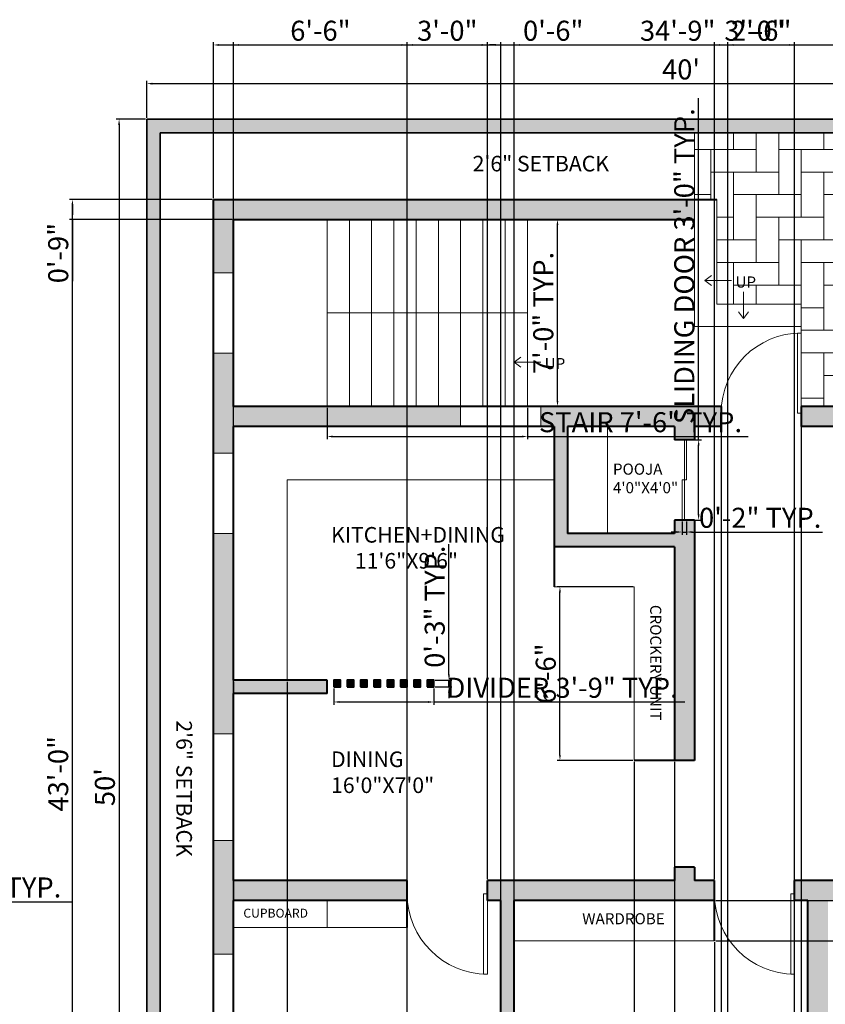
# Model space of a CAD drawing. Units: inches. Extents: x 2337 to 3570, y 1258 to 1938.
# Tile 21 of 30: x 2931 to 3293, y 1496 to 1938. Entities that reach past the tile are written whole.
import ezdxf

# ---------------------------------------------------------------- set-up
doc = ezdxf.new("R2010")
doc.units = ezdxf.units.IN
for name, color, linetype, lineweight in [('A-ANNO-DIMS', 2, 'Continuous', 18), ('A-ANNO-SYMB', 7, 'Continuous', 18), ('A-ANNO-TEXT', 7, 'Continuous', 18), ('A-AREA-IDEN', 7, 'Continuous', 18), ('A-DOOR', 4, 'Continuous', 20), ('A-FLOR-CASE', 34, 'Continuous', 18), ('A-FLOR-PATT', 252, 'Continuous', 13), ('A-FLOR-STRS', 7, 'Continuous', 20), ('A-GLAZ', 4, 'Continuous', 18), ('A-WALL', 7, 'Continuous', 40), ('C-PROP', 7, 'Continuous', 35)]:
    doc.layers.add(name, color=color, linetype=linetype, lineweight=lineweight)
doc.layers.add('A-WALL-PATT', color=18, linetype='Continuous', lineweight=13, true_color=0x000000)
doc.layers.add('C-PROP-PATT', color=251, linetype='Continuous', lineweight=13, true_color=0x636466)
doc.styles.get("Standard").update_dxf_attribs({"font": 'arial.ttf'})
doc.dimstyles.new('ISO-25', dxfattribs={"dimtxt": 9, "dimasz": 2.5, "dimexe": 1.25, "dimexo": 0.625, "dimtad": 1, "dimdec": 1, "dimlunit": 3, "dimtxsty": 'Standard', "dimcen": 2.5, "dimadec": 0, "dimazin": 0, "dimtfac": 1, "dimtdec": 1, "dimtmove": 0, "dimatfit": 3, "dimfxl": 1, "dimarcsym": 0})

# ---------------------------------------------------------------- blocks, each defined once
blk = doc.blocks.new('*U2')
for p, q in [((0, 0), (0, -6)), ((36, 0), (36, -6))]:
    blk.add_line(p, q)
blk.add_lwpolyline([(0, 0), (0, 36), (1.75, 36), (1.75, 0)], close=True)
blk.add_arc((0, 0), 36, 0, 90)
blk = doc.blocks.new('*D4')
at = {"layer": 'A-ANNO-DIMS', "color": 0, "lineweight": -2, "transparency": 16777216}
for p, q in [((2987.79, 1893.74), (2987.79, 1910.39)), ((2990.29, 1909.14), (3465.29, 1909.14)), ((3467.79, 1893.74), (3467.79, 1910.39))]:
    blk.add_line(p, q, dxfattribs=at)
at = {"layer": 'A-ANNO-DIMS', "color": 0, "transparency": 16777216}
for points in [[(2990.29, 1909.55), (2990.29, 1908.72), (2987.79, 1909.14)], [(3465.29, 1909.55), (3465.29, 1908.72), (3467.79, 1909.14)]]:
    blk.add_solid(points, dxfattribs=at)
at = {"layer": 'Defpoints', "color": 0, "transparency": 16777216}
for p in [(3467.79, 1909.14), (2987.79, 1893.12), (3467.79, 1893.12)]:
    blk.add_point(p, dxfattribs=at)
at = {"layer": 'A-ANNO-DIMS', "color": 0, "transparency": 16777216, "insert": (3227.79, 1914.36), "char_height": 9, "attachment_point": 5}
blk.add_mtext("40'", dxfattribs=at)
blk = doc.blocks.new('*D5')
at = {"layer": 'A-ANNO-DIMS', "color": 0, "lineweight": -2, "transparency": 16777216}
for p, q in [((2987.16, 1893.12), (2974.1, 1893.12)), ((2975.35, 1890.62), (2975.35, 1295.62)), ((2987.16, 1293.12), (2974.1, 1293.12))]:
    blk.add_line(p, q, dxfattribs=at)
at = {"layer": 'A-ANNO-DIMS', "color": 0, "transparency": 16777216}
for points in [[(2974.93, 1890.62), (2975.77, 1890.62), (2975.35, 1893.12)], [(2974.93, 1295.62), (2975.77, 1295.62), (2975.35, 1293.12)]]:
    blk.add_solid(points, dxfattribs=at)
at = {"layer": 'Defpoints', "color": 0, "transparency": 16777216}
for p in [(2987.79, 1893.12), (2975.35, 1293.12), (2987.79, 1293.12)]:
    blk.add_point(p, dxfattribs=at)
at = {"layer": 'A-ANNO-DIMS', "color": 0, "transparency": 16777216, "insert": (2970.13, 1593.12), "char_height": 9, "attachment_point": 5, "rotation": 90}
blk.add_mtext("50'", dxfattribs=at)
blk = doc.blocks.new('STAIR-UP-ARROW')
for p, q in [((2.25, 12), (2.25, 0)), ((2.25, 0), (0, 3.01)), ((2.25, 0), (4.5, 3.01))]:
    blk.add_line(p, q)
blk = doc.blocks.new('DOOR-SLIDING-36IN')
for p, q in [((1, 36), (1, 0)), ((2, 18), (2, 36)), ((1, 18), (0, 18)), ((0, 18), (0, 0)), ((1, 18), (2, 18))]:
    blk.add_line(p, q)
blk = doc.blocks.new('STAIR-DOUBLE-FLIGHT')
for p, q in [((0, 0), (0, 84)), ((10, 0), (10, 84)), ((20, 0), (20, 84)), ((30, 0), (30, 84)), ((40, 0), (40, 84)), ((50, 0), (50, 84)), ((60, 0), (60, 84)), ((70, 0), (70, 84)), ((80, 0), (80, 84)), ((90, 0), (90, 84)), ((0, 42), (90, 42))]:
    blk.add_line(p, q)
blk = doc.blocks.new('SCREEN-DIVIDER-8-POST')
h = blk.add_hatch(color=256)
h.dxf.hatch_style = 1
h.paths.add_polyline_path([(3, 3), (0, 3), (0, 0), (3, 0)])
h = blk.add_hatch(color=256)
h.dxf.hatch_style = 1
h.paths.add_polyline_path([(6, 3), (6, 0), (9, 0), (9, 3)])
h = blk.add_hatch(color=256)
h.dxf.hatch_style = 1
h.paths.add_polyline_path([(15, 3), (12, 3), (12, 0), (15, 0)])
h = blk.add_hatch(color=256)
h.dxf.hatch_style = 1
h.paths.add_polyline_path([(18, 3), (18, 0), (21, 0), (21, 3)])
h = blk.add_hatch(color=256)
h.dxf.hatch_style = 1
h.paths.add_polyline_path([(27, 3), (24, 3), (24, 0), (27, 0)])
h = blk.add_hatch(color=256)
h.dxf.hatch_style = 1
h.paths.add_polyline_path([(30, 3), (30, 0), (33, 0), (33, 3)])
h = blk.add_hatch(color=256)
h.dxf.hatch_style = 1
h.paths.add_polyline_path([(39, 3), (36, 3), (36, 0), (39, 0)])
h = blk.add_hatch(color=256)
h.dxf.hatch_style = 1
h.paths.add_polyline_path([(42, 3), (42, 0), (45, 0), (45, 3)])
for points in [[(0, 0), (3, 0), (3, 3), (0, 3)], [(6, 0), (9, 0), (9, 3), (6, 3)], [(12, 0), (15, 0), (15, 3), (12, 3)], [(18, 0), (21, 0), (21, 3), (18, 3)], [(24, 0), (27, 0), (27, 3), (24, 3)], [(30, 0), (33, 0), (33, 3), (30, 3)], [(36, 0), (39, 0), (39, 3), (36, 3)], [(42, 0), (45, 0), (45, 3), (42, 3)]]:
    blk.add_lwpolyline(points, close=True)
blk = doc.blocks.new('*D50')
at = {"layer": 'A-ANNO-DIMS', "color": 0, "lineweight": -2, "transparency": 16777216}
for p, q in [((2777.67, 1538.17), (2777.67, 1542.83)), ((2780.17, 1541.58), (2802.05, 1541.58)), ((2804.55, 1538.17), (2804.55, 1542.83)), ((2804.55, 1541.58), (2954.22, 1541.58))]:
    blk.add_line(p, q, dxfattribs=at)
at = {"layer": 'A-ANNO-DIMS', "color": 0, "transparency": 16777216}
for points in [[(2780.17, 1542), (2780.17, 1541.16), (2777.67, 1541.58)], [(2802.05, 1542), (2802.05, 1541.16), (2804.55, 1541.58)]]:
    blk.add_solid(points, dxfattribs=at)
at = {"layer": 'Defpoints', "color": 0, "transparency": 16777216}
for p in [(2804.55, 1541.58), (2777.67, 1537.55), (2804.55, 1537.55)]:
    blk.add_point(p, dxfattribs=at)
at = {"layer": 'A-ANNO-DIMS', "color": 0, "transparency": 16777216, "insert": (2880.63, 1546.87), "char_height": 9, "attachment_point": 5}
blk.add_mtext('PORCH CHAIR 2\'-3" TYP.', dxfattribs=at)
blk = doc.blocks.new('*D70')
at = {"layer": 'A-ANNO-DIMS', "color": 0, "lineweight": -2, "transparency": 16777216}
for p, q in [((3235.69, 1749.12), (3235.69, 1902.69)), ((3230.91, 1749.12), (3236.94, 1749.12)), ((3235.69, 1715.62), (3235.69, 1746.62)), ((3230.91, 1713.12), (3236.94, 1713.12))]:
    blk.add_line(p, q, dxfattribs=at)
at = {"layer": 'A-ANNO-DIMS', "color": 0, "transparency": 16777216}
for points in [[(3235.27, 1746.62), (3236.1, 1746.62), (3235.69, 1749.12)], [(3235.27, 1715.62), (3236.1, 1715.62), (3235.69, 1713.12)]]:
    blk.add_solid(points, dxfattribs=at)
at = {"layer": 'Defpoints', "color": 0, "transparency": 16777216}
for p in [(3230.29, 1749.12), (3235.69, 1749.12), (3230.29, 1713.12)]:
    blk.add_point(p, dxfattribs=at)
at = {"layer": 'A-ANNO-DIMS', "color": 0, "transparency": 16777216, "insert": (3230.4, 1827.15), "char_height": 9, "attachment_point": 5, "rotation": 90}
blk.add_mtext('SLIDING DOOR 3\'-0" TYP.', dxfattribs=at)
blk = doc.blocks.new('*D71')
at = {"layer": 'A-ANNO-DIMS', "color": 0, "lineweight": -2, "transparency": 16777216}
for p, q in [((3228.29, 1712.49), (3228.29, 1706.47)), ((3230.29, 1712.49), (3230.29, 1706.47)), ((3225.79, 1707.72), (3223.29, 1707.72)), ((3228.29, 1707.72), (3230.29, 1707.72)), ((3232.79, 1707.72), (3291.4, 1707.72))]:
    blk.add_line(p, q, dxfattribs=at)
at = {"layer": 'A-ANNO-DIMS', "color": 0, "transparency": 16777216}
for points in [[(3225.79, 1708.13), (3225.79, 1707.3), (3228.29, 1707.72)], [(3232.79, 1708.13), (3232.79, 1707.3), (3230.29, 1707.72)]]:
    blk.add_solid(points, dxfattribs=at)
at = {"layer": 'Defpoints', "color": 0, "transparency": 16777216}
for p in [(3228.29, 1713.12), (3230.29, 1713.12), (3230.29, 1707.72)]:
    blk.add_point(p, dxfattribs=at)
at = {"layer": 'A-ANNO-DIMS', "color": 0, "transparency": 16777216, "insert": (3263.34, 1712.94), "char_height": 9, "attachment_point": 5}
blk.add_mtext('0\'-2" TYP.', dxfattribs=at)
blk = doc.blocks.new('*D72')
at = {"layer": 'A-ANNO-DIMS', "color": 0, "lineweight": -2, "transparency": 16777216}
for p, q in [((3068.79, 1763.49), (3068.79, 1749.37)), ((3158.79, 1763.49), (3158.79, 1749.37)), ((3071.29, 1750.62), (3156.29, 1750.62)), ((3158.79, 1750.62), (3257.87, 1750.62))]:
    blk.add_line(p, q, dxfattribs=at)
at = {"layer": 'A-ANNO-DIMS', "color": 0, "transparency": 16777216}
for points in [[(3071.29, 1751.03), (3071.29, 1750.2), (3068.79, 1750.62)], [(3156.29, 1751.03), (3156.29, 1750.2), (3158.79, 1750.62)]]:
    blk.add_solid(points, dxfattribs=at)
at = {"layer": 'Defpoints', "color": 0, "transparency": 16777216}
for p in [(3068.79, 1764.12), (3158.79, 1764.12), (3158.79, 1750.62)]:
    blk.add_point(p, dxfattribs=at)
at = {"layer": 'A-ANNO-DIMS', "color": 0, "transparency": 16777216, "insert": (3209.58, 1755.89), "char_height": 9, "attachment_point": 5}
blk.add_mtext('STAIR 7\'-6" TYP.', dxfattribs=at)
blk = doc.blocks.new('*D73')
at = {"layer": 'A-ANNO-DIMS', "color": 0, "lineweight": -2, "transparency": 16777216}
for p, q in [((3159.41, 1848.12), (3173.54, 1848.12)), ((3172.29, 1766.62), (3172.29, 1845.62)), ((3159.41, 1764.12), (3173.54, 1764.12))]:
    blk.add_line(p, q, dxfattribs=at)
at = {"layer": 'A-ANNO-DIMS', "color": 0, "transparency": 16777216}
for points in [[(3171.87, 1845.62), (3172.7, 1845.62), (3172.29, 1848.12)], [(3171.87, 1766.62), (3172.7, 1766.62), (3172.29, 1764.12)]]:
    blk.add_solid(points, dxfattribs=at)
at = {"layer": 'Defpoints', "color": 0, "transparency": 16777216}
for p in [(3158.79, 1848.12), (3172.29, 1848.12), (3158.79, 1764.12)]:
    blk.add_point(p, dxfattribs=at)
at = {"layer": 'A-ANNO-DIMS', "color": 0, "transparency": 16777216, "insert": (3167.07, 1806.12), "char_height": 9, "attachment_point": 5, "rotation": 90}
blk.add_mtext('7\'-0" TYP.', dxfattribs=at)
blk = doc.blocks.new('*D76')
at = {"layer": 'A-ANNO-DIMS', "color": 0, "lineweight": -2, "transparency": 16777216}
for p, q in [((3071.79, 1637.49), (3071.79, 1630.12)), ((3116.79, 1637.49), (3116.79, 1630.12)), ((3074.29, 1631.37), (3114.29, 1631.37)), ((3116.79, 1631.37), (3229.44, 1631.37))]:
    blk.add_line(p, q, dxfattribs=at)
at = {"layer": 'A-ANNO-DIMS', "color": 0, "transparency": 16777216}
for points in [[(3074.29, 1631.78), (3074.29, 1630.95), (3071.79, 1631.37)], [(3114.29, 1631.78), (3114.29, 1630.95), (3116.79, 1631.37)]]:
    blk.add_solid(points, dxfattribs=at)
at = {"layer": 'Defpoints', "color": 0, "transparency": 16777216}
for p in [(3071.79, 1638.12), (3116.79, 1638.12), (3116.79, 1631.37)]:
    blk.add_point(p, dxfattribs=at)
at = {"layer": 'A-ANNO-DIMS', "color": 0, "transparency": 16777216, "insert": (3174.36, 1636.59), "char_height": 9, "attachment_point": 5}
blk.add_mtext('DIVIDER 3\'-9" TYP.', dxfattribs=at)
blk = doc.blocks.new('*D77')
at = {"layer": 'A-ANNO-DIMS', "color": 0, "lineweight": -2, "transparency": 16777216}
for p, q in [((3123.54, 1643.62), (3123.54, 1702.23)), ((3117.41, 1641.12), (3124.79, 1641.12)), ((3123.54, 1638.12), (3123.54, 1641.12)), ((3117.41, 1638.12), (3124.79, 1638.12)), ((3123.54, 1635.62), (3123.54, 1633.12))]:
    blk.add_line(p, q, dxfattribs=at)
at = {"layer": 'A-ANNO-DIMS', "color": 0, "transparency": 16777216}
for points in [[(3123.12, 1643.62), (3123.95, 1643.62), (3123.54, 1641.12)], [(3123.12, 1635.62), (3123.95, 1635.62), (3123.54, 1638.12)]]:
    blk.add_solid(points, dxfattribs=at)
at = {"layer": 'Defpoints', "color": 0, "transparency": 16777216}
for p in [(3116.79, 1641.12), (3123.54, 1641.12), (3116.79, 1638.12)]:
    blk.add_point(p, dxfattribs=at)
at = {"layer": 'A-ANNO-DIMS', "color": 0, "transparency": 16777216, "insert": (3118.31, 1674.17), "char_height": 9, "attachment_point": 5, "rotation": 90}
blk.add_mtext('0\'-3" TYP.', dxfattribs=at)
blk = doc.blocks.new('*D98')
at = {"layer": 'A-ANNO-DIMS', "color": 0, "lineweight": -2, "transparency": 16777216}
for p, q in [((3104.79, 1551.74), (3104.79, 1927.77)), ((3107.29, 1926.52), (3138.29, 1926.52)), ((3140.79, 1551.74), (3140.79, 1927.77))]:
    blk.add_line(p, q, dxfattribs=at)
at = {"layer": 'A-ANNO-DIMS', "color": 0, "transparency": 16777216}
for points in [[(3107.29, 1926.93), (3107.29, 1926.1), (3104.79, 1926.52)], [(3138.29, 1926.93), (3138.29, 1926.1), (3140.79, 1926.52)]]:
    blk.add_solid(points, dxfattribs=at)
at = {"layer": 'Defpoints', "color": 0, "transparency": 16777216}
for p in [(3140.79, 1926.52), (3104.79, 1551.12), (3140.79, 1551.12)]:
    blk.add_point(p, dxfattribs=at)
at = {"layer": 'A-ANNO-DIMS', "color": 0, "transparency": 16777216, "insert": (3122.79, 1931.74), "char_height": 9, "attachment_point": 5}
blk.add_mtext('3\'-0"', dxfattribs=at)
blk = doc.blocks.new('*D99')
at = {"layer": 'A-ANNO-DIMS', "color": 0, "lineweight": -2, "transparency": 16777216}
for p, q in [((3242.79, 1551.74), (3242.79, 1927.77)), ((3245.29, 1926.52), (3276.29, 1926.52)), ((3278.79, 1551.74), (3278.79, 1927.77))]:
    blk.add_line(p, q, dxfattribs=at)
at = {"layer": 'A-ANNO-DIMS', "color": 0, "transparency": 16777216}
for points in [[(3245.29, 1926.93), (3245.29, 1926.1), (3242.79, 1926.52)], [(3276.29, 1926.93), (3276.29, 1926.1), (3278.79, 1926.52)]]:
    blk.add_solid(points, dxfattribs=at)
at = {"layer": 'Defpoints', "color": 0, "transparency": 16777216}
for p in [(3278.79, 1926.52), (3242.79, 1551.12), (3278.79, 1551.12)]:
    blk.add_point(p, dxfattribs=at)
at = {"layer": 'A-ANNO-DIMS', "color": 0, "transparency": 16777216, "insert": (3260.79, 1931.74), "char_height": 9, "attachment_point": 5}
blk.add_mtext('3\'-0"', dxfattribs=at)
blk = doc.blocks.new('*D100')
at = {"layer": 'A-ANNO-DIMS', "color": 0, "lineweight": -2, "transparency": 16777216}
for p, q in [((3248.79, 1422.74), (3248.79, 1927.77)), ((3251.29, 1926.52), (3276.29, 1926.52)), ((3278.79, 1422.74), (3278.79, 1927.77))]:
    blk.add_line(p, q, dxfattribs=at)
at = {"layer": 'A-ANNO-DIMS', "color": 0, "transparency": 16777216}
for points in [[(3251.29, 1926.93), (3251.29, 1926.1), (3248.79, 1926.52)], [(3276.29, 1926.93), (3276.29, 1926.1), (3278.79, 1926.52)]]:
    blk.add_solid(points, dxfattribs=at)
at = {"layer": 'Defpoints', "color": 0, "transparency": 16777216}
for p in [(3278.79, 1926.52), (3248.79, 1422.12), (3278.79, 1422.12)]:
    blk.add_point(p, dxfattribs=at)
at = {"layer": 'A-ANNO-DIMS', "color": 0, "transparency": 16777216, "insert": (3263.79, 1931.74), "char_height": 9, "attachment_point": 5}
blk.add_mtext('2\'-6"', dxfattribs=at)
blk = doc.blocks.new('*D102')
at = {"layer": 'A-ANNO-DIMS', "color": 0, "lineweight": -2, "transparency": 16777216}
for p, q in [((3245.79, 1763.49), (3245.79, 1258.47)), ((3281.79, 1763.49), (3281.79, 1258.47)), ((3248.29, 1259.72), (3279.29, 1259.72))]:
    blk.add_line(p, q, dxfattribs=at)
at = {"layer": 'A-ANNO-DIMS', "color": 0, "transparency": 16777216}
for points in [[(3248.29, 1260.13), (3248.29, 1259.3), (3245.79, 1259.72)], [(3279.29, 1260.13), (3279.29, 1259.3), (3281.79, 1259.72)]]:
    blk.add_solid(points, dxfattribs=at)
at = {"layer": 'Defpoints', "color": 0, "transparency": 16777216}
for p in [(3245.79, 1764.12), (3281.79, 1764.12), (3281.79, 1259.72)]:
    blk.add_point(p, dxfattribs=at)
at = {"layer": 'A-ANNO-DIMS', "color": 0, "transparency": 16777216, "insert": (3263.79, 1264.94), "char_height": 9, "attachment_point": 5}
blk.add_mtext('3\'-0"', dxfattribs=at)
blk = doc.blocks.new('*D103')
at = {"layer": 'A-ANNO-DIMS', "color": 0, "lineweight": -2, "transparency": 16777216}
for p, q in [((3017.16, 1857.12), (2953.14, 1857.12)), ((2954.39, 1854.62), (2954.39, 1850.62)), ((3026.16, 1848.12), (2953.14, 1848.12)), ((2954.39, 1848.12), (2954.39, 1820.44))]:
    blk.add_line(p, q, dxfattribs=at)
at = {"layer": 'A-ANNO-DIMS', "color": 0, "transparency": 16777216}
for points in [[(2953.97, 1854.62), (2954.8, 1854.62), (2954.39, 1857.12)], [(2953.97, 1850.62), (2954.8, 1850.62), (2954.39, 1848.12)]]:
    blk.add_solid(points, dxfattribs=at)
at = {"layer": 'Defpoints', "color": 0, "transparency": 16777216}
for p in [(3017.79, 1857.12), (2954.39, 1848.12), (3026.79, 1848.12)]:
    blk.add_point(p, dxfattribs=at)
at = {"layer": 'A-ANNO-DIMS', "color": 0, "transparency": 16777216, "insert": (2949.17, 1833.03), "char_height": 9, "attachment_point": 5, "rotation": 90}
blk.add_mtext('0\'-9"', dxfattribs=at)
blk = doc.blocks.new('*D104')
at = {"layer": 'A-ANNO-DIMS', "color": 0, "lineweight": -2, "transparency": 16777216}
for p, q in [((3144.29, 1926.52), (3141.79, 1926.52)), ((3146.79, 1350.74), (3146.79, 1927.77)), ((3146.79, 1926.52), (3152.79, 1926.52)), ((3152.79, 1350.74), (3152.79, 1927.77)), ((3155.29, 1926.52), (3182.96, 1926.52))]:
    blk.add_line(p, q, dxfattribs=at)
at = {"layer": 'A-ANNO-DIMS', "color": 0, "transparency": 16777216}
for points in [[(3144.29, 1926.93), (3144.29, 1926.1), (3146.79, 1926.52)], [(3155.29, 1926.93), (3155.29, 1926.1), (3152.79, 1926.52)]]:
    blk.add_solid(points, dxfattribs=at)
at = {"layer": 'Defpoints', "color": 0, "transparency": 16777216}
for p in [(3152.79, 1926.52), (3146.79, 1350.12), (3152.79, 1350.12)]:
    blk.add_point(p, dxfattribs=at)
at = {"layer": 'A-ANNO-DIMS', "color": 0, "transparency": 16777216, "insert": (3170.37, 1931.74), "char_height": 9, "attachment_point": 5}
blk.add_mtext('0\'-6"', dxfattribs=at)
blk = doc.blocks.new('*D105')
at = {"layer": 'A-ANNO-DIMS', "color": 0, "lineweight": -2, "transparency": 16777216}
for p, q in [((3026.79, 1640.49), (3026.79, 1258.47)), ((3050.79, 1640.49), (3050.79, 1258.47)), ((3029.29, 1259.72), (3048.29, 1259.72)), ((3050.79, 1259.72), (3078.61, 1259.72))]:
    blk.add_line(p, q, dxfattribs=at)
at = {"layer": 'A-ANNO-DIMS', "color": 0, "transparency": 16777216}
for points in [[(3029.29, 1260.13), (3029.29, 1259.3), (3026.79, 1259.72)], [(3048.29, 1260.13), (3048.29, 1259.3), (3050.79, 1259.72)]]:
    blk.add_solid(points, dxfattribs=at)
at = {"layer": 'Defpoints', "color": 0, "transparency": 16777216}
for p in [(3026.79, 1641.12), (3050.79, 1641.12), (3050.79, 1259.72)]:
    blk.add_point(p, dxfattribs=at)
at = {"layer": 'A-ANNO-DIMS', "color": 0, "transparency": 16777216, "insert": (3065.95, 1264.94), "char_height": 9, "attachment_point": 5}
blk.add_mtext('2\'-0"', dxfattribs=at)
blk = doc.blocks.new('*D110')
at = {"layer": 'A-ANNO-DIMS', "color": 0, "lineweight": -2, "transparency": 16777216}
for p, q in [((3017.16, 1857.12), (2953.14, 1857.12)), ((2954.39, 1343.62), (2954.39, 1854.62)), ((3017.16, 1341.12), (2953.14, 1341.12))]:
    blk.add_line(p, q, dxfattribs=at)
at = {"layer": 'A-ANNO-DIMS', "color": 0, "transparency": 16777216}
for points in [[(2953.97, 1854.62), (2954.8, 1854.62), (2954.39, 1857.12)], [(2953.97, 1343.62), (2954.8, 1343.62), (2954.39, 1341.12)]]:
    blk.add_solid(points, dxfattribs=at)
at = {"layer": 'Defpoints', "color": 0, "transparency": 16777216}
for p in [(2954.39, 1857.12), (3017.79, 1857.12), (3017.79, 1341.12)]:
    blk.add_point(p, dxfattribs=at)
at = {"layer": 'A-ANNO-DIMS', "color": 0, "transparency": 16777216, "insert": (2949.16, 1599.12), "char_height": 9, "attachment_point": 5, "rotation": 90}
blk.add_mtext('43\'-0"', dxfattribs=at)
blk = doc.blocks.new('*D111')
at = {"layer": 'A-ANNO-DIMS', "color": 0, "lineweight": -2, "transparency": 16777216}
for p, q in [((3017.79, 1857.74), (3017.79, 1927.77)), ((3020.29, 1926.52), (3432.29, 1926.52)), ((3434.79, 1764.74), (3434.79, 1927.77))]:
    blk.add_line(p, q, dxfattribs=at)
at = {"layer": 'A-ANNO-DIMS', "color": 0, "transparency": 16777216}
for points in [[(3020.29, 1926.93), (3020.29, 1926.1), (3017.79, 1926.52)], [(3432.29, 1926.93), (3432.29, 1926.1), (3434.79, 1926.52)]]:
    blk.add_solid(points, dxfattribs=at)
at = {"layer": 'Defpoints', "color": 0, "transparency": 16777216}
for p in [(3434.79, 1926.52), (3017.79, 1857.12), (3434.79, 1764.12)]:
    blk.add_point(p, dxfattribs=at)
at = {"layer": 'A-ANNO-DIMS', "color": 0, "transparency": 16777216, "insert": (3226.29, 1931.74), "char_height": 9, "attachment_point": 5}
blk.add_mtext('34\'-9"', dxfattribs=at)
blk = doc.blocks.new('*D112')
at = {"layer": 'A-ANNO-DIMS', "color": 0, "lineweight": -2, "transparency": 16777216}
for p, q in [((3026.79, 1368.74), (3026.79, 1927.77)), ((3029.29, 1926.52), (3102.29, 1926.52)), ((3104.79, 1368.74), (3104.79, 1927.77))]:
    blk.add_line(p, q, dxfattribs=at)
at = {"layer": 'A-ANNO-DIMS', "color": 0, "transparency": 16777216}
for points in [[(3029.29, 1926.93), (3029.29, 1926.1), (3026.79, 1926.52)], [(3102.29, 1926.93), (3102.29, 1926.1), (3104.79, 1926.52)]]:
    blk.add_solid(points, dxfattribs=at)
at = {"layer": 'Defpoints', "color": 0, "transparency": 16777216}
for p in [(3104.79, 1926.52), (3026.79, 1368.12), (3104.79, 1368.12)]:
    blk.add_point(p, dxfattribs=at)
at = {"layer": 'A-ANNO-DIMS', "color": 0, "transparency": 16777216, "insert": (3065.79, 1931.74), "char_height": 9, "attachment_point": 5}
blk.add_mtext('6\'-6"', dxfattribs=at)
blk = doc.blocks.new('*D114')
at = {"layer": 'A-ANNO-DIMS', "color": 0, "lineweight": -2, "transparency": 16777216}
for p, q in [((3152.79, 1523.49), (3152.79, 1258.47)), ((3242.79, 1523.49), (3242.79, 1258.47)), ((3155.29, 1259.72), (3240.29, 1259.72))]:
    blk.add_line(p, q, dxfattribs=at)
at = {"layer": 'A-ANNO-DIMS', "color": 0, "transparency": 16777216}
for points in [[(3155.29, 1260.13), (3155.29, 1259.3), (3152.79, 1259.72)], [(3240.29, 1260.13), (3240.29, 1259.3), (3242.79, 1259.72)]]:
    blk.add_solid(points, dxfattribs=at)
at = {"layer": 'Defpoints', "color": 0, "transparency": 16777216}
for p in [(3152.79, 1524.12), (3242.79, 1524.12), (3242.79, 1259.72)]:
    blk.add_point(p, dxfattribs=at)
at = {"layer": 'A-ANNO-DIMS', "color": 0, "transparency": 16777216, "insert": (3197.79, 1264.94), "char_height": 9, "attachment_point": 5}
blk.add_mtext('7\'-6"', dxfattribs=at)
blk = doc.blocks.new('*D115')
at = {"layer": 'A-ANNO-DIMS', "color": 0, "lineweight": -2, "transparency": 16777216}
for p, q in [((3243.41, 1542.12), (3502.44, 1542.12)), ((3501.19, 1539.62), (3501.19, 1526.62)), ((3243.41, 1524.12), (3502.44, 1524.12)), ((3501.19, 1524.12), (3501.19, 1497.29))]:
    blk.add_line(p, q, dxfattribs=at)
at = {"layer": 'A-ANNO-DIMS', "color": 0, "transparency": 16777216}
for points in [[(3500.77, 1539.62), (3501.6, 1539.62), (3501.19, 1542.12)], [(3500.77, 1526.62), (3501.6, 1526.62), (3501.19, 1524.12)]]:
    blk.add_solid(points, dxfattribs=at)
at = {"layer": 'Defpoints', "color": 0, "transparency": 16777216}
for p in [(3242.79, 1542.12), (3242.79, 1524.12), (3501.19, 1524.12)]:
    blk.add_point(p, dxfattribs=at)
at = {"layer": 'A-ANNO-DIMS', "color": 0, "transparency": 16777216, "insert": (3495.97, 1509.45), "char_height": 9, "attachment_point": 5, "rotation": 90}
blk.add_mtext('1\'-6"', dxfattribs=at)
blk = doc.blocks.new('*D116')
at = {"layer": 'A-ANNO-DIMS', "color": 0, "lineweight": -2, "transparency": 16777216}
for p, q in [((3206.16, 1683.12), (3172.14, 1683.12)), ((3173.39, 1607.62), (3173.39, 1680.62)), ((3206.16, 1605.12), (3172.14, 1605.12))]:
    blk.add_line(p, q, dxfattribs=at)
at = {"layer": 'A-ANNO-DIMS', "color": 0, "transparency": 16777216}
for points in [[(3172.97, 1680.62), (3173.8, 1680.62), (3173.39, 1683.12)], [(3172.97, 1607.62), (3173.8, 1607.62), (3173.39, 1605.12)]]:
    blk.add_solid(points, dxfattribs=at)
at = {"layer": 'Defpoints', "color": 0, "transparency": 16777216}
for p in [(3173.39, 1683.12), (3206.79, 1683.12), (3206.79, 1605.12)]:
    blk.add_point(p, dxfattribs=at)
at = {"layer": 'A-ANNO-DIMS', "color": 0, "transparency": 16777216, "insert": (3168.17, 1644.12), "char_height": 9, "attachment_point": 5, "rotation": 90}
blk.add_mtext('6\'-6"', dxfattribs=at)
blk = doc.blocks.new('*D117')
at = {"layer": 'A-ANNO-DIMS', "color": 0, "lineweight": -2, "transparency": 16777216}
for p, q in [((3206.79, 1604.49), (3206.79, 1258.47)), ((3224.79, 1604.49), (3224.79, 1258.47)), ((3209.29, 1259.72), (3222.29, 1259.72)), ((3224.79, 1259.72), (3251.61, 1259.72))]:
    blk.add_line(p, q, dxfattribs=at)
at = {"layer": 'A-ANNO-DIMS', "color": 0, "transparency": 16777216}
for points in [[(3209.29, 1260.13), (3209.29, 1259.3), (3206.79, 1259.72)], [(3222.29, 1260.13), (3222.29, 1259.3), (3224.79, 1259.72)]]:
    blk.add_solid(points, dxfattribs=at)
at = {"layer": 'Defpoints', "color": 0, "transparency": 16777216}
for p in [(3206.79, 1605.12), (3224.79, 1605.12), (3224.79, 1259.72)]:
    blk.add_point(p, dxfattribs=at)
at = {"layer": 'A-ANNO-DIMS', "color": 0, "transparency": 16777216, "insert": (3239.45, 1264.94), "char_height": 9, "attachment_point": 5}
blk.add_mtext('1\'-6"', dxfattribs=at)

msp = doc.modelspace()

# ---------------------------------------------------------------- hatches: boundary and pattern name
at = {"layer": 'A-FLOR-PATT'}
h = msp.add_hatch(dxfattribs=at)
h.set_pattern_fill('AR-HBONE', color=256, scale=0.1, angle=45)
h.set_pattern_definition([(90, (-558.681, 0), (-10.16, 10.16), [30.48, -10.16]), (180, (-558.681, 10.16), (-10.16, 10.16), [30.48, -10.16])])
h.paths.add_polyline_path([(3281.79, 1810.12), (3281.79, 1764.12), (3434.79, 1764.12), (3461.79, 1764.12), (3461.79, 1779.12), (3464.79, 1779.12), (3464.79, 1875.12), (3461.79, 1875.12), (3461.79, 1887.12), (3233.79, 1887.12), (3233.79, 1857.12), (3243.79, 1857.12), (3243.79, 1810.12)])
h.paths.add_polyline_path([(3250.98, 1816.17), (3263.22, 1816.17), (3263.22, 1823.8), (3250.98, 1823.8)], flags=24)
h.paths.add_polyline_path([(3317.33, 1858.95), (3370.67, 1858.95), (3370.67, 1885.07), (3317.33, 1885.07)], flags=24)
at = {"layer": 'A-WALL-PATT'}
h = msp.add_hatch(color=256, dxfattribs=at)
h.dxf.hatch_style = 1
h.paths.add_polyline_path([(3233.79, 1857.12), (3017.79, 1857.12), (3017.79, 1824.12), (3026.79, 1824.12), (3026.79, 1848.12), (3233.79, 1848.12)])
h.paths.add_polyline_path([(3128.79, 1764.12), (3026.79, 1764.12), (3026.79, 1788.12), (3017.79, 1788.12), (3017.79, 1743.12), (3026.79, 1743.12), (3026.79, 1755.12), (3128.79, 1755.12)])
h.paths.add_polyline_path([(3245.79, 1761.12), (3245.79, 1764.12), (3164.79, 1764.12), (3164.79, 1755.12), (3170.79, 1755.12), (3170.79, 1701.12), (3224.79, 1701.12), (3224.79, 1605.12), (3233.79, 1605.12), (3233.79, 1713.12), (3224.79, 1713.12), (3224.79, 1707.12), (3176.79, 1707.12), (3176.79, 1755.12), (3224.79, 1755.12), (3224.79, 1749.12), (3233.79, 1749.12), (3233.79, 1755.12), (3245.79, 1755.12)])
h.paths.add_polyline_path([(3026.79, 1707.12), (3017.79, 1707.12), (3017.79, 1617.12), (3026.79, 1617.12), (3026.79, 1635.12), (3068.79, 1635.12), (3068.79, 1641.12), (3026.79, 1641.12)])
h.paths.add_polyline_path([(3104.79, 1551.12), (3026.79, 1551.12), (3026.79, 1569.12), (3017.79, 1569.12), (3017.79, 1518.12), (3026.79, 1518.12), (3026.79, 1542.12), (3104.79, 1542.12)])
h.paths.add_polyline_path([(3026.79, 1482.12), (3017.79, 1482.12), (3017.79, 1410.12), (3026.79, 1410.12)])
h.paths.add_polyline_path([(3188.79, 1350.12), (3152.79, 1350.12), (3152.79, 1380.12), (3146.79, 1380.12), (3146.79, 1350.12), (3026.79, 1350.12), (3026.79, 1374.12), (3017.79, 1374.12), (3017.79, 1341.12), (3188.79, 1341.12)])
h.paths.add_polyline_path([(3224.79, 1416.12), (3248.79, 1416.12), (3248.79, 1422.12), (3152.79, 1422.12), (3152.79, 1542.12), (3242.79, 1542.12), (3242.79, 1551.12), (3233.79, 1551.12), (3233.79, 1557.12), (3224.79, 1557.12), (3224.79, 1551.12), (3140.79, 1551.12), (3140.79, 1542.12), (3146.79, 1542.12), (3146.79, 1410.12), (3152.79, 1410.12), (3152.79, 1416.12), (3218.79, 1416.12), (3218.79, 1350.12), (3212.79, 1350.12), (3212.79, 1341.12), (3293.79, 1341.12), (3293.79, 1362.12), (3284.79, 1362.12), (3284.79, 1350.12), (3224.79, 1350.12)])
h.paths.add_polyline_path([(3293.79, 1434.12), (3284.79, 1434.12), (3284.79, 1422.12), (3278.79, 1422.12), (3278.79, 1416.12), (3284.79, 1416.12), (3284.79, 1386.12), (3293.79, 1386.12)], flags=17)
h.paths.add_polyline_path([(3293.79, 1542.12), (3314.79, 1542.12), (3314.79, 1551.12), (3278.79, 1551.12), (3278.79, 1545.12), (3278.79, 1542.12), (3284.79, 1542.12), (3284.79, 1482.12), (3293.79, 1482.12)])
h.paths.add_polyline_path([(3371.79, 1551.12), (3350.79, 1551.12), (3350.79, 1542.12), (3371.79, 1542.12), (3371.79, 1548.12)])
h.paths.add_polyline_path([(3434.79, 1647.12), (3425.79, 1647.12), (3425.79, 1551.12), (3419.79, 1551.12), (3419.79, 1548.12), (3419.79, 1542.12), (3434.79, 1542.12)])
h.paths.add_polyline_path([(3434.79, 1764.12), (3389.79, 1764.12), (3389.79, 1755.12), (3425.79, 1755.12), (3425.79, 1719.12), (3434.79, 1719.12)])
h.paths.add_polyline_path([(3317.79, 1764.12), (3281.79, 1764.12), (3281.79, 1755.12), (3317.79, 1755.12)])
at = {"layer": 'C-PROP-PATT'}
h = msp.add_hatch(color=256, dxfattribs=at)
h.dxf.hatch_style = 1
h.paths.add_polyline_path([(3467.79, 1893.12), (2987.79, 1893.12), (2987.79, 1293.12), (3293.79, 1293.12), (3293.79, 1299.12), (2993.79, 1299.12), (2993.79, 1887.12), (3461.79, 1887.12), (3461.79, 1875.12), (3467.79, 1875.12)])
h.paths.add_polyline_path([(3407.79, 1299.12), (3389.79, 1299.12), (3389.79, 1293.12), (3407.79, 1293.12)], flags=17)
h.paths.add_polyline_path([(3461.79, 1299.12), (3455.79, 1299.12), (3455.79, 1293.12), (3467.79, 1293.12), (3467.79, 1779.12), (3461.79, 1779.12)], flags=17)

# ---------------------------------------------------------------- linework, layer by layer
at = {"layer": 'A-FLOR-CASE'}
for p, q in [((3194.79, 1755.12), (3194.79, 1707.12)), ((3050.79, 1641.12), (3050.79, 1731.12)), ((3170.79, 1731.12), (3050.79, 1731.12)), ((3206.79, 1683.12), (3170.79, 1683.12)), ((3206.79, 1683.12), (3206.79, 1605.12)), ((3068.79, 1530.12), (3068.79, 1542.12)), ((3104.79, 1530.12), (3026.79, 1530.12)), ((3242.79, 1524.12), (3152.79, 1524.12))]:
    msp.add_line(p, q, dxfattribs=at)
at = {"layer": 'A-FLOR-STRS'}
for p, q in [((3233.79, 1887.12), (3233.79, 1800.12)), ((3243.79, 1857.12), (3243.79, 1810.12)), ((3281.79, 1810.12), (3243.79, 1810.12)), ((3281.79, 1764.12), (3281.79, 1810.12)), ((3281.79, 1800.12), (3233.79, 1800.12))]:
    msp.add_line(p, q, dxfattribs=at)
at = {"layer": 'A-GLAZ'}
for p, q in [((3026.79, 1824.12), (3017.79, 1824.12)), ((3026.79, 1788.12), (3017.79, 1788.12)), ((3128.79, 1764.12), (3128.79, 1755.12)), ((3164.79, 1764.12), (3164.79, 1755.12)), ((3026.79, 1743.12), (3017.79, 1743.12)), ((3026.79, 1707.12), (3017.79, 1707.12)), ((3026.79, 1617.12), (3017.79, 1617.12)), ((3026.79, 1569.12), (3017.79, 1569.12)), ((3026.79, 1518.12), (3017.79, 1518.12))]:
    msp.add_line(p, q, dxfattribs=at)
at = {"layer": 'A-WALL'}
for p, q in [((3017.79, 1857.12), (3243.79, 1857.12)), ((3017.79, 1341.12), (3017.79, 1857.12)), ((3026.79, 1848.12), (3233.79, 1848.12)), ((3026.79, 1764.12), (3026.79, 1848.12)), ((3245.79, 1764.12), (3026.79, 1764.12)), ((3245.79, 1764.12), (3245.79, 1755.12)), ((3434.79, 1764.12), (3281.79, 1764.12)), ((3281.79, 1764.12), (3281.79, 1755.12)), ((3026.79, 1641.12), (3026.79, 1755.12)), ((3170.79, 1755.12), (3026.79, 1755.12)), ((3170.79, 1755.12), (3170.79, 1683.12)), ((3176.79, 1755.12), (3176.79, 1707.12)), ((3224.79, 1755.12), (3176.79, 1755.12)), ((3224.79, 1755.12), (3224.79, 1749.12)), ((3233.79, 1755.12), (3233.79, 1749.12)), ((3245.79, 1755.12), (3233.79, 1755.12)), ((3425.79, 1755.12), (3281.79, 1755.12)), ((3233.79, 1749.12), (3224.79, 1749.12)), ((3233.79, 1713.12), (3224.79, 1713.12)), ((3224.79, 1713.12), (3224.79, 1707.12)), ((3233.79, 1713.12), (3233.79, 1605.12)), ((3224.79, 1707.12), (3176.79, 1707.12)), ((3224.79, 1701.12), (3170.79, 1701.12)), ((3224.79, 1701.12), (3224.79, 1605.12)), ((3068.79, 1641.12), (3026.79, 1641.12)), ((3068.79, 1635.12), (3068.79, 1641.12)), ((3026.79, 1551.12), (3026.79, 1635.12)), ((3068.79, 1635.12), (3026.79, 1635.12)), ((3233.79, 1605.12), (3206.79, 1605.12)), ((3233.79, 1557.12), (3224.79, 1557.12)), ((3224.79, 1557.12), (3224.79, 1551.12)), ((3233.79, 1557.12), (3233.79, 1551.12)), ((3104.79, 1551.12), (3026.79, 1551.12)), ((3104.79, 1530.12), (3104.79, 1551.12)), ((3224.79, 1551.12), (3140.79, 1551.12)), ((3140.79, 1542.12), (3140.79, 1551.12)), ((3242.79, 1551.12), (3233.79, 1551.12)), ((3242.79, 1524.12), (3242.79, 1551.12)), ((3278.79, 1542.12), (3278.79, 1551.12)), ((3371.79, 1551.12), (3278.79, 1551.12)), ((3026.79, 1350.12), (3026.79, 1542.12)), ((3104.79, 1542.12), (3026.79, 1542.12)), ((3146.79, 1542.12), (3140.79, 1542.12)), ((3146.79, 1410.12), (3146.79, 1542.12)), ((3152.79, 1422.12), (3152.79, 1542.12)), ((3242.79, 1542.12), (3152.79, 1542.12)), ((3284.79, 1542.12), (3278.79, 1542.12)), ((3284.79, 1422.12), (3284.79, 1542.12))]:
    msp.add_line(p, q, dxfattribs=at)
at = {"layer": 'C-PROP'}
for p, q in [((2987.79, 1893.12), (3467.79, 1893.12)), ((2987.79, 1293.12), (2987.79, 1893.12)), ((2993.79, 1299.12), (2993.79, 1887.12)), ((2993.79, 1887.12), (3461.79, 1887.12))]:
    msp.add_line(p, q, dxfattribs=at)

# ---------------------------------------------------------------- block references
at = {"layer": 'A-ANNO-SYMB'}
for p, rotation in [((3238.52, 1822.89), 270.0000000000029), ((3152.79, 1786.25), 270.0000000000043)]:
    msp.add_blockref('STAIR-UP-ARROW', p, dxfattribs=dict(at, rotation=rotation))
msp.add_blockref('STAIR-UP-ARROW', (3253.55, 1803.6), dxfattribs=at)
at = {"layer": 'A-DOOR', "xscale": -1}
msp.add_blockref('*U2', (3281.79, 1761.12), dxfattribs=at)
at = {"layer": 'A-DOOR'}
msp.add_blockref('DOOR-SLIDING-36IN', (3228.29, 1713.12), dxfattribs=at)
at = {"layer": 'A-DOOR', "rotation": 180}
for p in [(3140.79, 1545.12), (3278.79, 1545.12)]:
    msp.add_blockref('*U2', p, dxfattribs=at)
at = {"layer": 'A-FLOR-STRS'}
msp.add_blockref('STAIR-DOUBLE-FLIGHT', (3068.79, 1764.12), dxfattribs=at)
at = {"layer": 'A-WALL'}
msp.add_blockref('SCREEN-DIVIDER-8-POST', (3071.79, 1638.12), dxfattribs=at)

# ---------------------------------------------------------------- texts
at = {"layer": 'A-ANNO-TEXT'}
for p in [(3252.25, 1817.53), (3166.52, 1780.88)]:
    msp.add_text('UP', height=5, dxfattribs=at).set_placement(p)
at = {"layer": 'A-ANNO-TEXT', "attachment_point": 1}
for s, insert, char_height in [('2\'6" SETBACK', (3134.16, 1876.71), 7), ('CUPBOARD', (3031.17, 1538.51), 4), ('WARDROBE', (3183.39, 1536.5), 5)]:
    msp.add_mtext_dynamic_manual_height_columns(s, width=66.911, gutter_width=12.5, heights=[0], dxfattribs=dict(at, insert=insert, char_height=char_height))
at = {"layer": 'A-ANNO-TEXT', "attachment_point": 1, "rotation": 270}
for s, insert, char_height in [('CROCKERY UNIT', (3218.92, 1674.98), 5), ('2\'6" SETBACK', (3008.08, 1623.11), 7)]:
    msp.add_mtext_dynamic_manual_height_columns(s, width=66.911, gutter_width=12.5, heights=[0], dxfattribs=dict(at, insert=insert, char_height=char_height))
at = {"layer": 'A-AREA-IDEN', "attachment_point": 1}
for s, insert, char_height in [('POOJA\\P4\'0"X4\'0"', (3197.19, 1738.47), 5), ('KITCHEN+DINING\\P     11\'6"X9\'6"', (3070.56, 1709.96), 7), ('DINING\\P16\'0"X7\'0"', (3070.56, 1609.14), 7)]:
    msp.add_mtext_dynamic_manual_height_columns(s, width=66.911, gutter_width=12.5, heights=[0], dxfattribs=dict(at, insert=insert, char_height=char_height))

# ---------------------------------------------------------------- dimensions: what is measured, and where the dimension line sits
at = {"layer": 'A-ANNO-DIMS'}
for base, p1, p2, override, picture, middle in [((3434.79, 1926.52), (3017.79, 1857.12), (3434.79, 1764.12), {"dimdec": 1, "dimlfac": 1, "dimrnd": 0, "dimzin": 1, "dimdsep": 46, "dimlunit": 4, "dimfrac": 2}, '*D111', (3226.29, 1931.74)), ((3104.79, 1926.52), (3026.79, 1368.12), (3104.79, 1368.12), {"dimdec": 1, "dimlfac": 1, "dimrnd": 0, "dimzin": 1, "dimdsep": 46, "dimlunit": 4, "dimfrac": 2}, '*D112', (3065.79, 1931.74)), ((3140.79, 1926.52), (3104.79, 1551.12), (3140.79, 1551.12), {"dimdec": 1, "dimlfac": 1, "dimrnd": 0, "dimzin": 1, "dimdsep": 46, "dimlunit": 4, "dimfrac": 2}, '*D98', (3122.79, 1931.74)), ((3152.79, 1926.52), (3146.79, 1350.12), (3152.79, 1350.12), {"dimdec": 1, "dimlfac": 1, "dimrnd": 0, "dimzin": 1, "dimdsep": 46, "dimlunit": 4, "dimfrac": 2}, '*D104', (3170.37, 1931.74)), ((3278.79, 1926.52), (3242.79, 1551.12), (3278.79, 1551.12), {"dimdec": 1, "dimlfac": 1, "dimrnd": 0, "dimzin": 1, "dimdsep": 46, "dimlunit": 4, "dimfrac": 2}, '*D99', (3260.79, 1931.74)), ((3278.79, 1926.52), (3248.79, 1422.12), (3278.79, 1422.12), {"dimdec": 1, "dimlfac": 1, "dimrnd": 0, "dimzin": 1, "dimdsep": 46, "dimlunit": 4, "dimfrac": 2}, '*D100', (3263.79, 1931.74)), ((3467.79, 1909.14), (2987.79, 1893.12), (3467.79, 1893.12), {"dimclrd": 0, "dimclre": 0, "dimclrt": 0}, '*D4', (3227.79, 1914.36)), ((3281.79, 1259.72), (3245.79, 1764.12), (3281.79, 1764.12), {"dimdec": 1, "dimlfac": 1, "dimrnd": 0, "dimzin": 1, "dimdsep": 46, "dimlunit": 4, "dimfrac": 2}, '*D102', (3263.79, 1264.94)), ((3050.79, 1259.72), (3026.79, 1641.12), (3050.79, 1641.12), {"dimdec": 1, "dimlfac": 1, "dimrnd": 0, "dimzin": 1, "dimdsep": 46, "dimlunit": 4, "dimfrac": 2}, '*D105', (3065.95, 1264.94)), ((3224.79, 1259.72), (3206.79, 1605.12), (3224.79, 1605.12), {"dimdec": 1, "dimlfac": 1, "dimrnd": 0, "dimzin": 1, "dimdsep": 46, "dimlunit": 4, "dimfrac": 2}, '*D117', (3239.45, 1264.94)), ((3242.79, 1259.72), (3152.79, 1524.12), (3242.79, 1524.12), {"dimdec": 1, "dimlfac": 1, "dimrnd": 0, "dimzin": 1, "dimdsep": 46, "dimlunit": 4, "dimfrac": 2}, '*D114', (3197.79, 1264.94))]:
    dim = msp.add_linear_dim(base=base, p1=p1, p2=p2, dimstyle='ISO-25', override=override, dxfattribs=at)
    dim.commit()
    dim.dimension.update_dxf_attribs({"geometry": picture, "text_midpoint": middle})
for base, p1, p2, text, picture, middle in [((3235.69, 1749.12), (3230.29, 1713.12), (3230.29, 1749.12), 'SLIDING DOOR <> TYP.', '*D70', (3230.4, 1827.15)), ((3172.29, 1848.12), (3158.79, 1764.12), (3158.79, 1848.12), '<> TYP.', '*D73', (3167.07, 1806.12)), ((3123.54, 1641.12), (3116.79, 1638.12), (3116.79, 1641.12), '<> TYP.', '*D77', (3118.31, 1674.17))]:
    dim = msp.add_linear_dim(base=base, p1=p1, p2=p2, angle=90, text=text, dimstyle='ISO-25', override={"dimdec": 1, "dimlfac": 1, "dimrnd": 0, "dimzin": 1, "dimdsep": 46, "dimlunit": 4, "dimfrac": 2}, dxfattribs=at)
    dim.commit()
    dim.dimension.update_dxf_attribs({"geometry": picture, "text_midpoint": middle})
for base, p1, p2, override, picture, middle in [((2975.35, 1293.12), (2987.79, 1893.12), (2987.79, 1293.12), {"dimclrd": 0, "dimclre": 0, "dimclrt": 0}, '*D5', (2970.13, 1593.12)), ((2954.39, 1848.12), (3017.79, 1857.12), (3026.79, 1848.12), {"dimdec": 1, "dimlfac": 1, "dimrnd": 0, "dimzin": 1, "dimdsep": 46, "dimlunit": 4, "dimfrac": 2}, '*D103', (2949.17, 1833.03)), ((2954.39, 1857.12), (3017.79, 1341.12), (3017.79, 1857.12), {"dimdec": 1, "dimlfac": 1, "dimrnd": 0, "dimzin": 1, "dimdsep": 46, "dimlunit": 4, "dimfrac": 2}, '*D110', (2949.16, 1599.12)), ((3173.39, 1683.12), (3206.79, 1605.12), (3206.79, 1683.12), {"dimdec": 1, "dimlfac": 1, "dimrnd": 0, "dimzin": 1, "dimdsep": 46, "dimlunit": 4, "dimfrac": 2}, '*D116', (3168.17, 1644.12)), ((3501.19, 1524.12), (3242.79, 1542.12), (3242.79, 1524.12), {"dimdec": 1, "dimlfac": 1, "dimrnd": 0, "dimzin": 1, "dimdsep": 46, "dimlunit": 4, "dimfrac": 2}, '*D115', (3495.97, 1509.45))]:
    dim = msp.add_linear_dim(base=base, p1=p1, p2=p2, angle=90, dimstyle='ISO-25', override=override, dxfattribs=at)
    dim.commit()
    dim.dimension.update_dxf_attribs({"geometry": picture, "text_midpoint": middle})
for base, p1, p2, text, picture, middle in [((3158.79, 1750.62), (3068.79, 1764.12), (3158.79, 1764.12), 'STAIR <> TYP.', '*D72', (3209.58, 1755.89)), ((3230.29, 1707.72), (3228.29, 1713.12), (3230.29, 1713.12), '<> TYP.', '*D71', (3263.34, 1712.94)), ((3116.79, 1631.37), (3071.79, 1638.12), (3116.79, 1638.12), 'DIVIDER <> TYP.', '*D76', (3174.36, 1636.59)), ((2804.55, 1541.58), (2777.67, 1537.55), (2804.55, 1537.55), 'PORCH CHAIR <> TYP.', '*D50', (2880.63, 1546.87))]:
    dim = msp.add_linear_dim(base=base, p1=p1, p2=p2, text=text, dimstyle='ISO-25', override={"dimdec": 1, "dimlfac": 1, "dimrnd": 0, "dimzin": 1, "dimdsep": 46, "dimlunit": 4, "dimfrac": 2}, dxfattribs=at)
    dim.commit()
    dim.dimension.update_dxf_attribs({"geometry": picture, "text_midpoint": middle})

doc.saveas('drawing.dxf')
